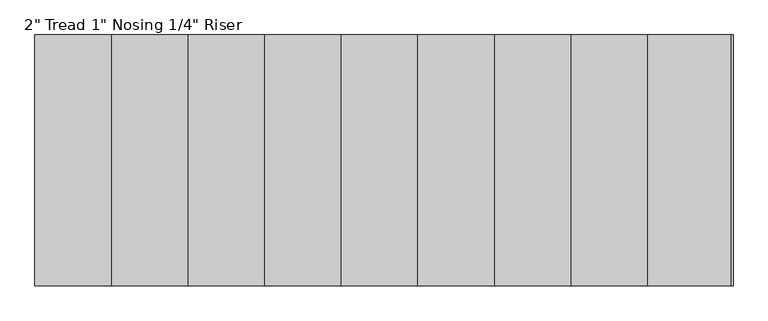
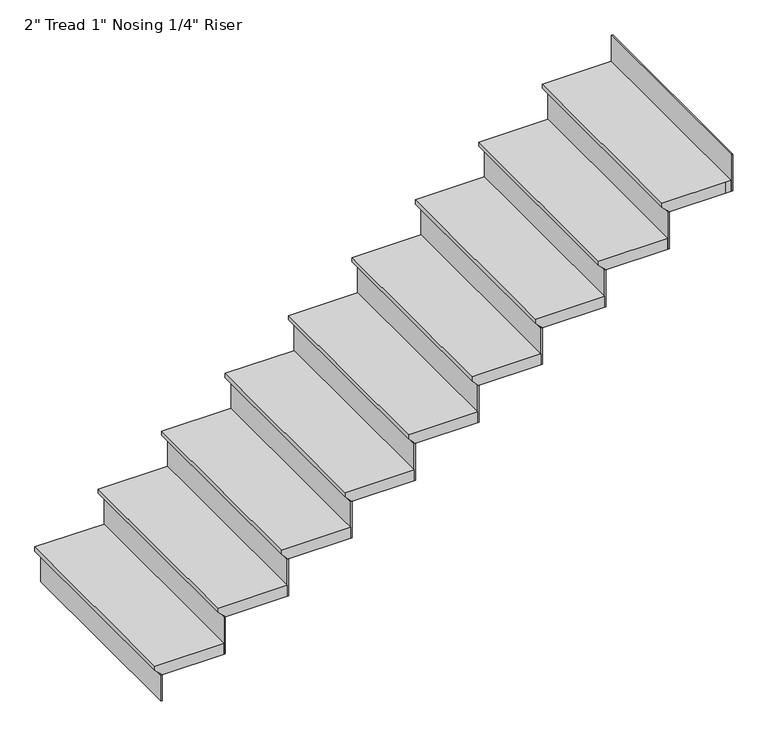
"""IFC4 building model written with IfcOpenShell, lengths in millimetres: stair flight geometry."""

from ifc_helpers import new_model, si_unit, origin, place, context, project, spatial, faceted_brep, source, transform, mapped, element, save


def stair_flight_f1cb69c7(model_context):
    return source(origin(), model_context, "Body", "Brep", [
        faceted_brep([(-8269.5911408, -6224.7337491, 457.2), (-8269.5911408, -6224.7337491, 476.25), (-8269.5911408, -5310.3337491, 476.25), (-8269.5911408, -5310.3337491, 457.2), (-8244.1911408, -6224.7337491, 431.8), (-8244.1911408, -5310.3337491, 431.8), (-7964.7911408, -6224.7337491, 476.25), (-7964.7911408, -5310.3337491, 476.25), (-8244.1911408, -5310.3337491, 425.45), (-7964.7911408, -5310.3337491, 425.45), (-7964.7911408, -6224.7337491, 425.45), (-8244.1911408, -6224.7337491, 425.45)], [[[0, 1, 2, 3]], [[4, 0, 3, 5]], [[2, 1, 6, 7]], [[8, 9, 10, 11]], [[2, 7, 9, 8, 5, 3]], [[8, 11, 4, 5]], [[6, 1, 0, 4, 11, 10]], [[7, 6, 10, 9]]]),
        faceted_brep([(-8244.1911408, -6224.7337491, 425.45), (-8244.1911408, -6224.7337491, 304.8), (-8237.8411408, -6224.7337491, 304.8), (-8237.8411408, -6224.7337491, 425.45), (-8244.1911408, -5310.3337491, 425.45), (-8237.8411408, -5310.3337491, 425.45), (-8237.8411408, -5310.3337491, 304.8), (-8244.1911408, -5310.3337491, 304.8)], [[[0, 1, 2, 3]], [[4, 5, 6, 7]], [[1, 0, 4, 7]], [[2, 1, 7, 6]], [[3, 2, 6, 5]], [[0, 3, 5, 4]]]),
        faceted_brep([(-7964.7911408, -6224.7337491, 596.9), (-7964.7911408, -6224.7337491, 425.45), (-7958.4411408, -6224.7337491, 425.45), (-7958.4411408, -6224.7337491, 596.9), (-7964.7911408, -5310.3337491, 596.9), (-7958.4411408, -5310.3337491, 596.9), (-7958.4411408, -5310.3337491, 425.45), (-7964.7911408, -5310.3337491, 425.45)], [[[0, 1, 2, 3]], [[4, 5, 6, 7]], [[1, 0, 4, 7]], [[2, 1, 7, 6]], [[3, 2, 6, 5]], [[0, 3, 5, 4]]]),
        faceted_brep([(-7990.1911408, -5310.3337491, 647.7), (-7990.1911408, -6224.7337491, 647.7), (-7685.3911408, -6224.7337491, 647.7), (-7685.3911408, -5310.3337491, 647.7), (-7964.7911408, -5310.3337491, 596.9), (-7685.3911408, -5310.3337491, 596.9), (-7685.3911408, -6224.7337491, 596.9), (-7964.7911408, -6224.7337491, 596.9), (-7964.7911408, -5310.3337491, 603.25), (-7990.1911408, -5310.3337491, 628.65), (-7964.7911408, -6224.7337491, 603.25), (-7990.1911408, -6224.7337491, 628.65)], [[[0, 1, 2, 3]], [[4, 5, 6, 7]], [[0, 3, 5, 4, 8, 9]], [[4, 7, 10, 8]], [[2, 1, 11, 10, 7, 6]], [[3, 2, 6, 5]], [[11, 1, 0, 9]], [[10, 11, 9, 8]]]),
        faceted_brep([(-7685.3911408, -6224.7337491, 768.35), (-7685.3911408, -6224.7337491, 596.9), (-7679.0411408, -6224.7337491, 596.9), (-7679.0411408, -6224.7337491, 768.35), (-7685.3911408, -5310.3337491, 768.35), (-7679.0411408, -5310.3337491, 768.35), (-7679.0411408, -5310.3337491, 596.9), (-7685.3911408, -5310.3337491, 596.9)], [[[0, 1, 2, 3]], [[4, 5, 6, 7]], [[1, 0, 4, 7]], [[2, 1, 7, 6]], [[3, 2, 6, 5]], [[0, 3, 5, 4]]]),
        faceted_brep([(-7710.7911408, -5310.3337491, 819.15), (-7710.7911408, -6224.7337491, 819.15), (-7405.9911408, -6224.7337491, 819.15), (-7405.9911408, -5310.3337491, 819.15), (-7685.3911408, -5310.3337491, 768.35), (-7405.9911408, -5310.3337491, 768.35), (-7405.9911408, -6224.7337491, 768.35), (-7685.3911408, -6224.7337491, 768.35), (-7685.3911408, -5310.3337491, 774.7), (-7710.7911408, -5310.3337491, 800.1), (-7685.3911408, -6224.7337491, 774.7), (-7710.7911408, -6224.7337491, 800.1)], [[[0, 1, 2, 3]], [[4, 5, 6, 7]], [[0, 3, 5, 4, 8, 9]], [[4, 7, 10, 8]], [[2, 1, 11, 10, 7, 6]], [[3, 2, 6, 5]], [[11, 1, 0, 9]], [[10, 11, 9, 8]]]),
        faceted_brep([(-7405.9911408, -6224.7337491, 939.8), (-7405.9911408, -6224.7337491, 768.35), (-7399.6411408, -6224.7337491, 768.35), (-7399.6411408, -6224.7337491, 939.8), (-7405.9911408, -5310.3337491, 939.8), (-7399.6411408, -5310.3337491, 939.8), (-7399.6411408, -5310.3337491, 768.35), (-7405.9911408, -5310.3337491, 768.35)], [[[0, 1, 2, 3]], [[4, 5, 6, 7]], [[1, 0, 4, 7]], [[2, 1, 7, 6]], [[3, 2, 6, 5]], [[0, 3, 5, 4]]]),
        faceted_brep([(-7431.3911408, -5310.3337491, 990.6), (-7431.3911408, -6224.7337491, 990.6), (-7126.5911408, -6224.7337491, 990.6), (-7126.5911408, -5310.3337491, 990.6), (-7405.9911408, -5310.3337491, 939.8), (-7126.5911408, -5310.3337491, 939.8), (-7126.5911408, -6224.7337491, 939.8), (-7405.9911408, -6224.7337491, 939.8), (-7405.9911408, -5310.3337491, 946.15), (-7431.3911408, -5310.3337491, 971.55), (-7405.9911408, -6224.7337491, 946.15), (-7431.3911408, -6224.7337491, 971.55)], [[[0, 1, 2, 3]], [[4, 5, 6, 7]], [[0, 3, 5, 4, 8, 9]], [[4, 7, 10, 8]], [[2, 1, 11, 10, 7, 6]], [[3, 2, 6, 5]], [[11, 1, 0, 9]], [[10, 11, 9, 8]]]),
        faceted_brep([(-7126.5911408, -6224.7337491, 1111.25), (-7126.5911408, -6224.7337491, 939.8), (-7120.2411408, -6224.7337491, 939.8), (-7120.2411408, -6224.7337491, 1111.25), (-7126.5911408, -5310.3337491, 1111.25), (-7120.2411408, -5310.3337491, 1111.25), (-7120.2411408, -5310.3337491, 939.8), (-7126.5911408, -5310.3337491, 939.8)], [[[0, 1, 2, 3]], [[4, 5, 6, 7]], [[1, 0, 4, 7]], [[2, 1, 7, 6]], [[3, 2, 6, 5]], [[0, 3, 5, 4]]]),
        faceted_brep([(-7151.9911408, -5310.3337491, 1162.05), (-7151.9911408, -6224.7337491, 1162.05), (-6847.1911408, -6224.7337491, 1162.05), (-6847.1911408, -5310.3337491, 1162.05), (-7126.5911408, -5310.3337491, 1111.25), (-6847.1911408, -5310.3337491, 1111.25), (-6847.1911408, -6224.7337491, 1111.25), (-7126.5911408, -6224.7337491, 1111.25), (-7126.5911408, -5310.3337491, 1117.6), (-7151.9911408, -5310.3337491, 1143.0), (-7126.5911408, -6224.7337491, 1117.6), (-7151.9911408, -6224.7337491, 1143.0)], [[[0, 1, 2, 3]], [[4, 5, 6, 7]], [[0, 3, 5, 4, 8, 9]], [[4, 7, 10, 8]], [[2, 1, 11, 10, 7, 6]], [[3, 2, 6, 5]], [[11, 1, 0, 9]], [[10, 11, 9, 8]]]),
        faceted_brep([(-6847.1911408, -6224.7337491, 1282.7), (-6847.1911408, -6224.7337491, 1111.25), (-6840.8411408, -6224.7337491, 1111.25), (-6840.8411408, -6224.7337491, 1282.7), (-6847.1911408, -5310.3337491, 1282.7), (-6840.8411408, -5310.3337491, 1282.7), (-6840.8411408, -5310.3337491, 1111.25), (-6847.1911408, -5310.3337491, 1111.25)], [[[0, 1, 2, 3]], [[4, 5, 6, 7]], [[1, 0, 4, 7]], [[2, 1, 7, 6]], [[3, 2, 6, 5]], [[0, 3, 5, 4]]]),
        faceted_brep([(-6872.5911408, -5310.3337491, 1333.5), (-6872.5911408, -6224.7337491, 1333.5), (-6567.7911408, -6224.7337491, 1333.5), (-6567.7911408, -5310.3337491, 1333.5), (-6847.1911408, -5310.3337491, 1282.7), (-6567.7911408, -5310.3337491, 1282.7), (-6567.7911408, -6224.7337491, 1282.7), (-6847.1911408, -6224.7337491, 1282.7), (-6847.1911408, -5310.3337491, 1289.05), (-6872.5911408, -5310.3337491, 1314.45), (-6847.1911408, -6224.7337491, 1289.05), (-6872.5911408, -6224.7337491, 1314.45)], [[[0, 1, 2, 3]], [[4, 5, 6, 7]], [[0, 3, 5, 4, 8, 9]], [[4, 7, 10, 8]], [[2, 1, 11, 10, 7, 6]], [[3, 2, 6, 5]], [[11, 1, 0, 9]], [[10, 11, 9, 8]]]),
        faceted_brep([(-6567.7911408, -6224.7337491, 1454.15), (-6567.7911408, -6224.7337491, 1282.7), (-6561.4411408, -6224.7337491, 1282.7), (-6561.4411408, -6224.7337491, 1454.15), (-6567.7911408, -5310.3337491, 1454.15), (-6561.4411408, -5310.3337491, 1454.15), (-6561.4411408, -5310.3337491, 1282.7), (-6567.7911408, -5310.3337491, 1282.7)], [[[0, 1, 2, 3]], [[4, 5, 6, 7]], [[1, 0, 4, 7]], [[2, 1, 7, 6]], [[3, 2, 6, 5]], [[0, 3, 5, 4]]]),
        faceted_brep([(-6593.1911408, -5310.3337491, 1504.95), (-6593.1911408, -6224.7337491, 1504.95), (-6288.3911408, -6224.7337491, 1504.95), (-6288.3911408, -5310.3337491, 1504.95), (-6567.7911408, -5310.3337491, 1454.15), (-6288.3911408, -5310.3337491, 1454.15), (-6288.3911408, -6224.7337491, 1454.15), (-6567.7911408, -6224.7337491, 1454.15), (-6567.7911408, -5310.3337491, 1460.5), (-6593.1911408, -5310.3337491, 1485.9), (-6567.7911408, -6224.7337491, 1460.5), (-6593.1911408, -6224.7337491, 1485.9)], [[[0, 1, 2, 3]], [[4, 5, 6, 7]], [[0, 3, 5, 4, 8, 9]], [[4, 7, 10, 8]], [[2, 1, 11, 10, 7, 6]], [[3, 2, 6, 5]], [[11, 1, 0, 9]], [[10, 11, 9, 8]]]),
        faceted_brep([(-6288.3911408, -6224.7337491, 1625.6), (-6288.3911408, -6224.7337491, 1454.15), (-6282.0411408, -6224.7337491, 1454.15), (-6282.0411408, -6224.7337491, 1625.6), (-6288.3911408, -5310.3337491, 1625.6), (-6282.0411408, -5310.3337491, 1625.6), (-6282.0411408, -5310.3337491, 1454.15), (-6288.3911408, -5310.3337491, 1454.15)], [[[0, 1, 2, 3]], [[4, 5, 6, 7]], [[1, 0, 4, 7]], [[2, 1, 7, 6]], [[3, 2, 6, 5]], [[0, 3, 5, 4]]]),
        faceted_brep([(-6313.7911408, -5310.3337491, 1676.4), (-6313.7911408, -6224.7337491, 1676.4), (-6008.9911408, -6224.7337491, 1676.4), (-6008.9911408, -5310.3337491, 1676.4), (-6288.3911408, -5310.3337491, 1625.6), (-6008.9911408, -5310.3337491, 1625.6), (-6008.9911408, -6224.7337491, 1625.6), (-6288.3911408, -6224.7337491, 1625.6), (-6288.3911408, -5310.3337491, 1631.95), (-6313.7911408, -5310.3337491, 1657.35), (-6288.3911408, -6224.7337491, 1631.95), (-6313.7911408, -6224.7337491, 1657.35)], [[[0, 1, 2, 3]], [[4, 5, 6, 7]], [[0, 3, 5, 4, 8, 9]], [[4, 7, 10, 8]], [[2, 1, 11, 10, 7, 6]], [[3, 2, 6, 5]], [[11, 1, 0, 9]], [[10, 11, 9, 8]]]),
        faceted_brep([(-5729.5911408, -6224.7337491, 1968.5), (-5729.5911408, -6224.7337491, 1797.05), (-5723.2411408, -6224.7337491, 1797.05), (-5723.2411408, -6224.7337491, 1968.5), (-5729.5911408, -5310.3337491, 1968.5), (-5723.2411408, -5310.3337491, 1968.5), (-5723.2411408, -5310.3337491, 1797.05), (-5729.5911408, -5310.3337491, 1797.05)], [[[0, 1, 2, 3]], [[4, 5, 6, 7]], [[1, 0, 4, 7]], [[2, 1, 7, 6]], [[3, 2, 6, 5]], [[0, 3, 5, 4]]]),
        faceted_brep([(-6008.9911408, -6224.7337491, 1797.05), (-6008.9911408, -6224.7337491, 1625.6), (-6002.6411408, -6224.7337491, 1625.6), (-6002.6411408, -6224.7337491, 1797.05), (-6008.9911408, -5310.3337491, 1797.05), (-6002.6411408, -5310.3337491, 1797.05), (-6002.6411408, -5310.3337491, 1625.6), (-6008.9911408, -5310.3337491, 1625.6)], [[[0, 1, 2, 3]], [[4, 5, 6, 7]], [[1, 0, 4, 7]], [[2, 1, 7, 6]], [[3, 2, 6, 5]], [[0, 3, 5, 4]]]),
        faceted_brep([(-5729.5911408, -5310.3337491, 1847.85), (-5754.9911408, -5310.3337491, 1847.85), (-6034.3911408, -5310.3337491, 1847.85), (-6034.3911408, -6224.7337491, 1847.85), (-5754.9911408, -6224.7337491, 1847.85), (-5729.5911408, -6224.7337491, 1847.85), (-5754.9911408, -5310.3337491, 1797.05), (-5729.5911408, -5310.3337491, 1797.05), (-5729.5911408, -6224.7337491, 1797.05), (-5754.9911408, -6224.7337491, 1797.05), (-6008.9911408, -6224.7337491, 1797.05), (-6008.9911408, -5310.3337491, 1797.05), (-6008.9911408, -5310.3337491, 1803.4), (-6034.3911408, -5310.3337491, 1828.8), (-6008.9911408, -6224.7337491, 1803.4), (-6034.3911408, -6224.7337491, 1828.8)], [[[0, 1, 2, 3, 4, 5]], [[6, 7, 8, 9, 10, 11]], [[1, 0, 7, 6]], [[2, 1, 6, 11, 12, 13]], [[11, 10, 14, 12]], [[4, 3, 15, 14, 10, 9]], [[5, 4, 9, 8]], [[0, 5, 8, 7]], [[15, 3, 2, 13]], [[14, 15, 13, 12]]]),
    ])


if __name__ == "__main__":
    model = new_model("IFC4")
    model_context = context("Model", 3, world=origin())
    ifc_project = project(units=[si_unit("LENGTHUNIT", "METRE", prefix="MILLI")], contexts=[model_context])
    site = spatial("IfcSite", under=ifc_project)
    building = spatial("IfcBuilding", under=site)
    placement = place(None, origin())
    stair_flight_shape = stair_flight_f1cb69c7(model_context)
    element("IfcStairFlight", 1, ObjectType="2\" Tread 1\" Nosing 1/4\" Riser", at=placement, inside=building, context=model_context, shape_type="MappedRepresentation", body=[
        mapped(stair_flight_shape, transform((0.0, 0.0, 0.0), x_axis=(1.0, 0.0, 0.0), y_axis=(0.0, 1.0, 0.0), z_axis=(0.0, 0.0, 1.0))),
    ])
    save(model, "model.ifc")
